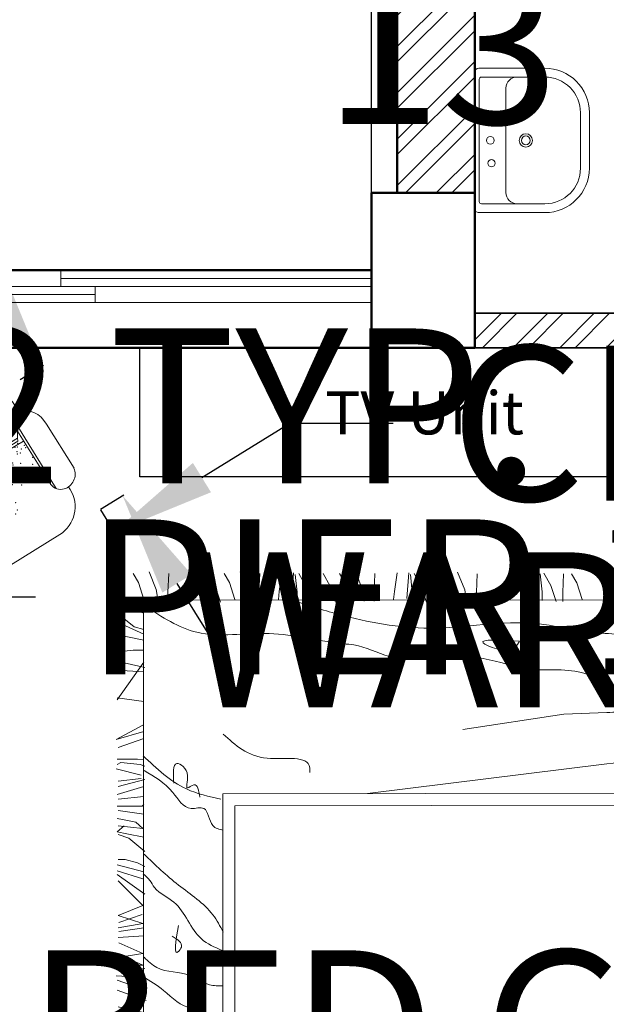
# Model space of a CAD drawing. Units: inches. Extents: x -90 to 536, y -553 to 299.
# Tile 19 of 27: x 69 to 137, y 58 to 173. Entities that reach past the tile are written whole.
import ezdxf

# ---------------------------------------------------------------- set-up
doc = ezdxf.new("R2010")
doc.units = ezdxf.units.IN
for name, color, linetype, lineweight in [('A-ANNO-DIMS', 2, 'Continuous', 18), ('A-ANNO-TEXT', 7, 'Continuous', 18), ('A-COLS', 7, 'Continuous', 50), ('A-FLOR-CASE', 2, 'Continuous', 25), ('A-FLOR-FIXT', 8, 'Continuous', 18), ('A-GLAZ', 4, 'Continuous', 18), ('A-WALL-PATT', 252, 'Continuous', 13), ('Furniture', 2, 'Continuous', 18), ('Inner Wall', 5, 'Continuous', 35), ('Outer Wall', 1, 'Continuous', 50)]:
    doc.layers.add(name, color=color, linetype=linetype, lineweight=lineweight)
doc.styles.get("Standard").update_dxf_attribs({"font": 'arial.ttf'})
doc.dimstyles.get("Standard").update_dxf_attribs({"dimtxt": 18, "dimasz": 12, "dimexe": 0.18, "dimexo": 0.0625, "dimgap": 0.09, "dimtad": 0, "dimtih": 1, "dimtoh": 1, "dimdec": 0, "dimzin": 0, "dimdsep": 46, "dimlunit": 3, "dimtxsty": 'Standard', "dimcen": 0.09, "dimadec": 0, "dimazin": 0, "dimtfac": 1, "dimtdec": 0, "dimtofl": 0, "dimtmove": 0, "dimatfit": 3, "dimfxl": 1, "dimtolj": 1, "dimtzin": 0, "dimarcsym": 0})

# ---------------------------------------------------------------- blocks, each defined once
blk = doc.blocks.new('A$C57EA129C')
for p, q in [((0, 0.4428), (0, 0.1782)), ((0.016, 0.4589), (0.5631, 0.4589)), ((0.0445, 0.441), (0.5346, 0.441)), ((0.5791, 0.4428), (0.5791, 0.1782)), ((0.0356, 0.4321), (0.0356, 0.2896)), ((0.5435, 0.4321), (0.5435, 0.2896)), ((0.0802, 0.3341), (0.499, 0.3341)), ((0.0356, 0.2896), (0.0356, 0.1782)), ((0.5435, 0.2896), (0.5435, 0.1782)), ((0.1782, 0.0356), (0.4009, 0.0356)), ((0.1782, 0), (0.4009, 0))]:
    blk.add_line(p, q)
for centre, radius in [((0.1982, 0.392), 0.0143), ((0.2896, 0.3965), 0.0156), ((0.3809, 0.392), 0.0143), ((0.2896, 0.2545), 0.0267), ((0.2896, 0.2545), 0.0178)]:
    blk.add_circle(centre, radius)
for centre, radius, start, end in [((0.016, 0.4428), 0.016, 90, 180), ((0.0445, 0.4321), 0.00891, 90, 180), ((0.5346, 0.4321), 0.00891, 0, 90), ((0.5631, 0.4428), 0.016, 0, 90), ((0.0802, 0.2896), 0.0445, 90, 180), ((0.499, 0.2896), 0.0445, 0, 90), ((0.1782, 0.1782), 0.1782, 180, 270), ((0.1782, 0.1782), 0.1426, 180, 270), ((0.4009, 0.1782), 0.1782, 270, 0), ((0.4009, 0.1782), 0.1426, 270, 0)]:
    blk.add_arc(centre, radius, start, end)
blk = doc.blocks.new('A$C14440869')
for p, q in [((299.4, 786.8), (654.5, 786.8)), ((141.1, 259.3), (141.1, 621.8)), ((154.9, 258.1), (156.1, 601.9)), ((799, 258.1), (797.7, 601.9)), ((812.8, 224.7), (812.8, 621.8)), ((0, 267.1), (1, 551.8)), ((798, 537.4), (157.2, 552.6)), ((953.9, 267.1), (952.8, 551.8)), ((78.7, 198), (78.7, 179.8)), ((875.1, 196.3), (875.2, 179.8)), ((257.3, 0.1), (696.7, 0))]:
    blk.add_line(p, q)
for centre, radius, start, end in [((178, 741.7), 84.9, 46.4058, 190.9946), ((775.9, 741.7), 84.9, 349.0054, 133.5942), ((490.5, 1647.2), 881.3, 253.2515, 257.4746), ((463.3, 1647.2), 881.3, 282.5254, 286.7485), ((146, 557.8), 145.1, 108.7163, 182.3743), ((810.8, 559.8), 142.3, 356.766, 72.1434), ((234.9, -29958.2), 30532.1, 88.98134, 90.11086), ((164.3, -28909.7), 29469.6, 88.82111, 89.96326), ((79.9, 278.7), 80.7, 188.2473, 288.8842), ((90.3, 265.5), 65, 283.9696, 353.4821), ((871.6, 268.6), 73.4, 188.2144, 251.9677), ((869.8, 281.5), 85.3, 255.8372, 350.3327), ((257.8, 179.2), 179.2, 179.795, 269.795), ((696, 179.2), 179.2, 270.205, 0.205)]:
    blk.add_arc(centre, radius, start, end)
for points in [[(94.6, 725.5), (94.6, 660.2), (167.2, 599.5), (183.2, 559.8)], [(859.3, 725.5), (859.3, 660.2), (786.7, 599.5), (770.6, 553.6)]]:
    blk.add_open_spline(points, degree=3)
for p in [(261.8, 540.6), (346.3, 540.6), (358.4, 564.7), (446.9, 540.6), (467, 548.6), (656.1, 560.7), (692.1, 540.6), (752.6, 568.7), (764.7, 544.6), (201.4, 528.5), (294, 500.4), (302, 528.5), (306.1, 524.5), (346.3, 496.4), (386.5, 484.3), (446.9, 496.4), (454.9, 524.5), (487.1, 516.5), (507.2, 520.5), (531.4, 496.4), (595.7, 520.5), (603.8, 520.5), (603.8, 484.3), (647.8, 524.5), (651.8, 528.5), (656.1, 532.5), (656.1, 524.5), (659.9, 500.4), (688.3, 492.3), (696.3, 520.5), (700.3, 528.5), (732.5, 496.4), (736.6, 508.4), (740.6, 532.5), (748.6, 492.3), (752.4, 528.5), (764.7, 508.4), (788.9, 516.5), (788.9, 500.4), (233.6, 444.1), (294, 456.2), (334.2, 444.1), (378.5, 456.2), (454.9, 480.3), (479.1, 456.2), (487.1, 440.1), (519.3, 432.1), (539.4, 480.3), (543.4, 480.3), (571.6, 472.3), (659.9, 456.2), (680.2, 456.2), (684.2, 468.2), (720.2, 444.1), (792.9, 436.1), (181.3, 403.9), (326.2, 416), (692.3, 383.9), (772.5, 403.9), (181.3, 335.6), (225.6, 339.6), (290, 339.6), (418.7, 327.6), (619.9, 367.8), (663.9, 339.6), (728.3, 339.6), (772.5, 335.6), (776.8, 339.6), (229.6, 315.5), (326.2, 303.5), (583.7, 275.4), (724.3, 315.5), (551.5, 223.1), (571.6, 235.2), (334.2, 215.1)]:
    blk.add_point(p)
blk = doc.blocks.new('A$C2B723114')
for p, q in [((0, 2.9047), (2.8274, 2.9047)), ((0, 2.8487), (0, 2.9047)), ((2.8274, 2.9047), (2.8274, 2.8487)), ((0.4243, 2.8697), (0.4243, 2.4855)), ((2.4742, 2.8697), (2.4742, 2.4855)), ((2.8274, 2.8487), (0, 2.8487)), ((0.1012, 2.4649), (0.1012, 2.849)), ((0.1396, 2.5033), (0.1396, 2.849)), ((0.6794, 0.7051), (0.6794, 2.8509)), ((0.7187, 0.7435), (0.7187, 2.8509)), ((2.1776, 2.8509), (2.1776, 0.7454)), ((2.216, 2.8509), (2.216, 0.707)), ((2.6798, 2.5052), (2.6798, 2.8509)), ((2.7182, 2.4668), (2.7182, 2.8509)), ((0.6087, 2.6776), (0.295, 2.6776)), ((2.6586, 2.6776), (2.2821, 2.6776)), ((1.3789, 2.4999), (1.3598, 2.5761)), ((2.0593, 2.4999), (2.0402, 2.5761)), ((0.6766, 2.5033), (0.1396, 2.5033)), ((1.3858, 2.4723), (1.3789, 2.4999)), ((2.0662, 2.4723), (2.0593, 2.4999)), ((2.2188, 2.5052), (2.6798, 2.5052)), ((0.6794, 2.4649), (0.1012, 2.4649)), ((0.7191, 2.47), (2.1778, 2.4719)), ((2.2188, 2.4668), (2.7182, 2.4668)), ((2.1771, 2.3036), (0.718, 2.1685)), ((1.0365, 1.6233), (2.1246, 2.2989)), ((2.2287, 1.6076), (2.2523, 1.5035)), ((0.5047, 1.5819), (0.5353, 1.4945)), ((0.6174, 1.5819), (0.6232, 1.4916)), ((0.6467, 1.5819), (0.6369, 1.5137)), ((0.6571, 1.4945), (0.6571, 1.5765)), ((2.2726, 1.593), (2.3061, 1.5007)), ((2.3067, 1.5881), (2.3373, 1.5007)), ((2.4194, 1.5881), (2.4251, 1.4979)), ((2.4487, 1.5881), (2.4389, 1.5199)), ((2.4591, 1.5007), (2.4591, 1.5828)), ((0.4269, 0.0884), (0.4269, 1.4945)), ((0.4269, 1.4945), (0.6794, 1.4945)), ((2.4685, 1.4964), (2.216, 1.5022)), ((2.4685, 1.4964), (2.4685, 0.0903)), ((0.3172, 1.3923), (0.4213, 1.3687)), ((2.4685, 1.4044), (2.5491, 1.3861)), ((2.4596, 1.3659), (2.552, 1.3324)), ((0.3318, 1.3485), (0.4241, 1.3149)), ((2.4645, 1.3318), (2.552, 1.3012)), ((0.3367, 1.3143), (0.4241, 1.2838)), ((2.4645, 1.2928), (2.5548, 1.2871)), ((2.4645, 1.2635), (2.5328, 1.2733)), ((2.4699, 1.2531), (2.552, 1.2163)), ((2.552, 1.2531), (2.4699, 1.2531)), ((2.5435, 1.2276), (2.4699, 1.2163)), ((0.3367, 1.2016), (0.427, 1.1959)), ((2.4699, 1.2163), (2.5463, 1.1823)), ((0.3367, 1.1724), (0.405, 1.1821)), ((0.4241, 1.162), (0.3421, 1.162)), ((0.3421, 1.162), (0.4241, 1.1252)), ((2.5491, 1.1654), (2.467, 1.1597)), ((2.5463, 1.1455), (2.467, 1.1342)), ((2.5491, 1.1342), (2.4699, 1.1201)), ((2.4699, 1.1201), (2.5491, 1.0946)), ((2.5463, 1.1172), (2.4727, 1.0918)), ((2.5491, 1.0946), (2.4699, 1.0635)), ((2.4699, 1.0635), (2.5491, 0.9842)), ((0.4157, 1.0206), (0.3421, 1.0093)), ((0.3421, 1.0093), (0.4185, 0.9754)), ((2.4642, 1.0267), (2.552, 0.9644)), ((2.4699, 0.9785), (2.552, 0.9531)), ((0.4213, 0.9584), (0.3392, 0.9527)), ((2.467, 0.9559), (2.552, 0.9333)), ((0.4185, 0.9386), (0.3392, 0.9272)), ((0.4213, 0.9272), (0.3421, 0.9131)), ((0.3421, 0.9131), (0.4213, 0.8876)), ((0.4185, 0.9103), (0.3449, 0.8848)), ((2.4642, 0.9389), (2.4869, 0.9276)), ((2.4869, 0.9276), (2.5265, 0.9163)), ((2.5265, 0.9163), (2.5491, 0.9163)), ((0.4213, 0.8876), (0.3421, 0.8565)), ((2.4642, 0.8908), (2.5152, 0.8483)), ((0.3421, 0.8565), (0.4213, 0.7772)), ((2.5152, 0.8483), (2.5491, 0.837)), ((0.3364, 0.8197), (0.4241, 0.7574)), ((2.467, 0.8455), (2.5208, 0.8342)), ((2.4699, 0.8172), (2.4925, 0.7974)), ((2.5491, 0.8087), (2.4699, 0.8172)), ((2.5208, 0.8342), (2.552, 0.8285)), ((2.552, 0.8285), (2.5293, 0.8087)), ((2.4925, 0.7974), (2.535, 0.7889)), ((2.535, 0.7889), (2.552, 0.7861)), ((0.3421, 0.7716), (0.4241, 0.7461)), ((2.5491, 0.7606), (2.467, 0.7719)), ((0.3392, 0.7489), (0.4241, 0.7263)), ((2.1776, 0.7454), (0.7187, 0.7435)), ((2.4727, 0.7464), (2.467, 0.7408)), ((2.467, 0.7153), (2.5491, 0.7238)), ((2.552, 0.7464), (2.4727, 0.7464)), ((0.359, 0.7206), (0.3987, 0.7093)), ((0.3987, 0.7093), (0.4213, 0.7093)), ((2.216, 0.707), (0.6794, 0.7051)), ((0.9938, 0.6115), (1.7555, 0.7064)), ((2.552, 0.7096), (2.467, 0.6842)), ((0.3421, 0.6601), (0.4213, 0.5808)), ((2.5491, 0.6842), (2.4642, 0.6615)), ((2.5491, 0.6672), (2.4755, 0.6587)), ((2.4755, 0.6474), (2.5548, 0.6276)), ((0.3364, 0.6233), (0.4241, 0.561)), ((2.4642, 0.6191), (2.4784, 0.6134)), ((2.467, 0.5993), (2.4869, 0.5964)), ((2.4784, 0.6134), (2.5406, 0.6077)), ((2.4869, 0.5964), (2.552, 0.5964)), ((2.5406, 0.6077), (2.552, 0.6134)), ((0.3421, 0.5752), (0.4241, 0.5497)), ((0.3392, 0.5525), (0.4241, 0.5299)), ((2.467, 0.5313), (2.5491, 0.5596)), ((2.467, 0.5087), (2.5548, 0.5342)), ((2.5548, 0.5342), (2.4699, 0.4889)), ((0.359, 0.5242), (0.3987, 0.5129)), ((1.4523, 0.5021), (1.1305, 0.4537)), ((0.3364, 0.4785), (0.3874, 0.436)), ((1.1305, 0.4537), (0.9938, 0.448)), ((0.4213, 0.415), (0.3364, 0.3923)), ((0.3392, 0.4332), (0.393, 0.4219)), ((0.4241, 0.2868), (0.3392, 0.415)), ((0.3874, 0.436), (0.4213, 0.4247)), ((0.393, 0.4219), (0.4241, 0.4162)), ((0.4241, 0.4162), (0.4015, 0.3964)), ((2.467, 0.4133), (2.552, 0.4019)), ((0.3421, 0.4049), (0.3647, 0.3851)), ((0.4213, 0.3964), (0.3421, 0.4049)), ((0.4213, 0.398), (0.3477, 0.3895)), ((0.3647, 0.3851), (0.4072, 0.3766)), ((0.4072, 0.3766), (0.4241, 0.3738)), ((2.467, 0.2879), (2.552, 0.4076)), ((0.4213, 0.3377), (0.3392, 0.3491)), ((0.4241, 0.3236), (0.3449, 0.3236)), ((2.467, 0.319), (2.5548, 0.3134)), ((0.3392, 0.2925), (0.4213, 0.3009)), ((2.4642, 0.3049), (2.5491, 0.2851)), ((0.3477, 0.2571), (0.427, 0.2373)), ((2.501, 0.2491), (2.5491, 0.2547)), ((0.3506, 0.2231), (0.4128, 0.2175)), ((0.4128, 0.2175), (0.4241, 0.2231)), ((2.4699, 0.2491), (2.501, 0.2491)), ((0.359, 0.2061), (0.4241, 0.2061)), ((2.467, 0.2179), (2.5605, 0.1981)), ((2.467, 0.1981), (2.5491, 0.1613)), ((2.467, 0.184), (2.4982, 0.1755)), ((2.4982, 0.1755), (2.5463, 0.1359)), ((0.3392, 0.1042), (0.4213, 0.1325)), ((2.4699, 0.1302), (2.535, 0.1104)), ((0.3392, 0.0815), (0.427, 0.107)), ((0.427, 0.107), (0.3421, 0.0617)), ((0.7334, 0.0943), (0.7503, 0.0434)), ((0.956, 0.0943), (0.973, 0.0434)), ((1.1542, 0.0943), (1.1712, 0.0434)), ((1.5674, 0.0962), (1.5844, 0.0453)), ((1.8568, 0.0962), (1.8738, 0.0453)), ((1.9342, 0.0962), (1.9512, 0.0453)), ((2.2236, 0.0962), (2.2406, 0.0453)), ((2.4642, 0.0991), (2.5378, 0.0877)), ((2.535, 0.1104), (2.5491, 0.0991)), ((2.4685, 0.0903), (0.4269, 0.0884)), ((0.5106, 0.0657), (0.5077, 0.0063)), ((0.5106, 0.094), (0.5106, 0.0657)), ((0.5417, 0.094), (0.5474, 0.0572)), ((0.587, 0.0884), (0.604, 0.0346)), ((0.6512, 0.0884), (0.6682, 0.0346)), ((0.713, 0.0657), (0.7101, 0.0063)), ((0.713, 0.094), (0.713, 0.0657)), ((0.7786, 0.0915), (0.7786, 0.0632)), ((0.7786, 0.0632), (0.7843, 0.0066)), ((0.8739, 0.0884), (0.8908, 0.0346)), ((1.0013, 0.0915), (1.0013, 0.0632)), ((1.0013, 0.0632), (1.007, 0.0066)), ((1.072, 0.0884), (1.089, 0.0346)), ((1.1338, 0.0657), (1.131, 0.0063)), ((1.1338, 0.094), (1.1338, 0.0657)), ((1.1995, 0.0915), (1.1995, 0.0632)), ((1.1995, 0.0632), (1.2052, 0.0066)), ((1.4088, 0.0657), (1.406, 0.0063)), ((1.4088, 0.094), (1.4088, 0.0657)), ((1.44, 0.094), (1.4456, 0.0572)), ((1.4853, 0.0884), (1.5023, 0.0346)), ((1.6127, 0.0934), (1.6127, 0.0651)), ((1.6127, 0.0651), (1.6184, 0.0085)), ((1.6297, 0.0849), (1.624, 0.0028)), ((1.6721, 0.0877), (1.6693, 0.0623)), ((1.7344, 0.0651), (1.7316, 0.0057)), ((1.7344, 0.0934), (1.7344, 0.0651)), ((1.7655, 0.0934), (1.7712, 0.0566)), ((1.8108, 0.0877), (1.8278, 0.034)), ((1.9795, 0.0934), (1.9795, 0.0651)), ((1.9795, 0.0651), (1.9852, 0.0085)), ((1.9965, 0.0849), (1.9908, 0.0028)), ((2.039, 0.0877), (2.0361, 0.0623)), ((2.1012, 0.0651), (2.0984, 0.0057)), ((2.1012, 0.0934), (2.1012, 0.0651)), ((2.1324, 0.0934), (2.138, 0.0566)), ((2.1777, 0.0877), (2.1946, 0.034)), ((2.2689, 0.0934), (2.2689, 0.0651)), ((2.2689, 0.0651), (2.2746, 0.0085)), ((2.2859, 0.0849), (2.2802, 0.0028)), ((2.3284, 0.0877), (2.3255, 0.0623)), ((2.3906, 0.0651), (2.3878, 0.0057)), ((2.3906, 0.0934), (2.3906, 0.0651)), ((2.4218, 0.0934), (2.4274, 0.0566)), ((2.467, 0.0877), (2.484, 0.034)), ((2.5378, 0.0877), (2.5463, 0.0821)), ((0.5474, 0.0572), (0.57, 0.0006)), ((0.604, 0.0346), (0.621, 0.0063)), ((0.6682, 0.0346), (0.6851, 0.0063)), ((0.7503, 0.0434), (0.773, 0.0037)), ((0.8908, 0.0346), (0.9078, 0.0063)), ((0.973, 0.0434), (0.9957, 0.0037)), ((1.089, 0.0346), (1.106, 0.0063)), ((1.1712, 0.0434), (1.1939, 0.0037)), ((1.4456, 0.0572), (1.4683, 0.0006)), ((1.5023, 0.0346), (1.5192, 0.0082)), ((1.5844, 0.0453), (1.607, 0.0057)), ((1.6693, 0.0623), (1.6608, 0.0028)), ((1.7712, 0.0566), (1.7938, 0)), ((1.8278, 0.034), (1.8448, 0.0057)), ((1.8738, 0.0453), (1.8964, 0.0057)), ((1.9512, 0.0453), (1.9739, 0.0057)), ((2.0361, 0.0623), (2.0276, 0.0028)), ((2.138, 0.0566), (2.1607, 0)), ((2.1946, 0.034), (2.2116, 0.0057)), ((2.2406, 0.0453), (2.2632, 0.0057)), ((2.3255, 0.0623), (2.317, 0.0028)), ((2.4274, 0.0566), (2.4501, 0)), ((2.484, 0.034), (2.501, 0.0057))]:
    blk.add_line(p, q)
for centre, radius in [((0.4243, 2.6776), 0.0821), ((2.4742, 2.6776), 0.0821), ((0.4243, 2.6776), 0.0493), ((2.4742, 2.6776), 0.0493)]:
    blk.add_circle(centre, radius)
for centre, radius, start, end in [((0.8088, 2.8207), 0.00315, 111.7883, 160.436), ((0.8162, 2.8021), 0.0232, 94.3025, 111.7883), ((0.8165, 2.7987), 0.0266, 59.3487, 94.3025), ((1.4892, 2.8207), 0.00315, 111.7883, 160.436), ((1.4966, 2.8021), 0.0232, 94.3025, 111.7883), ((1.4969, 2.7987), 0.0266, 59.3487, 94.3025), ((0.8078, 2.821), 0.00214, 160.436, 281.8931), ((0.8091, 2.8151), 0.00394, 21.9904, 101.8931), ((0.8409, 2.7949), 0.0302, 158.579, 188.1335), ((0.7994, 2.8112), 0.0144, 338.579, 21.9904), ((0.8554, 2.8643), 0.0497, 239.3487, 264.7408), ((0.9202, 3.5684), 0.7568, 264.7408, 268.0921), ((0.8679, 2.7254), 0.0915, 74.0648, 94.2159), ((0.8679, 2.7254), 0.0915, 53.9136, 74.0648), ((0.9409, 4.189), 1.3777, 268.0921, 270.5757), ((0.8679, 2.7254), 0.0915, 36.1766, 53.9136), ((0.86, 2.6097), 0.2158, 62.7604, 69.1397), ((0.9466, 3.6164), 0.8051, 270.5757, 274.8018), ((0.9263, 2.7386), 0.0708, 51.6114, 62.7604), ((0.7461, 2.511), 0.3611, 46.1885, 51.6114), ((1.0364, 2.548), 0.2671, 87.4614, 94.8018), ((1.042, 2.6745), 0.1405, 79.8101, 87.4614), ((1.1532, 3.2931), 0.488, 259.8101, 263.9133), ((1.204, 3.7695), 0.9671, 263.9133, 270), ((1.204, 3.4318), 0.6294, 270, 277.5469), ((1.2573, 3.0292), 0.2233, 277.5469, 285.744), ((1.3941, 2.5438), 0.281, 98.4372, 105.744), ((1.3747, 2.6748), 0.1486, 90, 98.4372), ((1.3713, 2.8186), 0.0315, 274.4002, 333.4195), ((1.3747, 2.74), 0.0833, 78.7276, 90), ((1.3886, 2.8099), 0.0121, 333.4195, 78.7276), ((1.4882, 2.821), 0.00214, 160.436, 281.8931), ((1.4895, 2.8151), 0.00394, 21.9904, 101.8931), ((1.5213, 2.7949), 0.0302, 158.579, 188.1335), ((1.4798, 2.8112), 0.0144, 338.579, 21.9904), ((1.5358, 2.8643), 0.0497, 239.3487, 264.7408), ((1.6006, 3.5684), 0.7568, 264.7408, 268.0921), ((1.5483, 2.7254), 0.0915, 74.0648, 94.2159), ((1.5483, 2.7254), 0.0915, 53.9136, 74.0648), ((1.6213, 4.189), 1.3777, 268.0921, 270.5757), ((1.5483, 2.7254), 0.0915, 36.1766, 53.9136), ((1.5404, 2.6097), 0.2158, 62.7604, 69.1397), ((1.627, 3.6164), 0.8051, 270.5757, 274.8018), ((1.6067, 2.7386), 0.0708, 51.6114, 62.7604), ((1.4265, 2.511), 0.3611, 46.1885, 51.6114), ((1.7168, 2.548), 0.2671, 87.4614, 94.8018), ((1.7224, 2.6745), 0.1405, 79.8101, 87.4614), ((1.8336, 3.2931), 0.488, 259.8101, 263.9133), ((1.8844, 3.7695), 0.9671, 263.9133, 270), ((1.8844, 3.4318), 0.6294, 270, 277.5469), ((1.9377, 3.0292), 0.2233, 277.5469, 285.744), ((2.0745, 2.5438), 0.281, 98.4372, 105.744), ((2.0551, 2.6748), 0.1486, 90, 98.4372), ((2.0517, 2.8186), 0.0315, 274.4002, 333.4195), ((2.0551, 2.74), 0.0833, 78.7276, 90), ((2.069, 2.8099), 0.0121, 333.4195, 78.7276), ((1.0356, 2.8227), 0.2268, 188.1335, 192.1095), ((0.635, 2.7368), 0.1829, 7.6809, 12.1095), ((-0.0181, 2.6487), 0.8418, 3.3687, 7.6809), ((0.8679, 2.7254), 0.0915, 18.4397, 36.1766), ((0.8523, 2.6218), 0.2076, 39.0349, 46.1885), ((0.923, 2.7382), 0.4535, 0, 6.2324), ((1.716, 2.8227), 0.2268, 188.1335, 192.1095), ((1.3154, 2.7368), 0.1829, 7.6809, 12.1095), ((0.6623, 2.6487), 0.8418, 3.3687, 7.6809), ((1.5483, 2.7254), 0.0915, 18.4397, 36.1766), ((1.5327, 2.6218), 0.2076, 39.0349, 46.1885), ((1.6034, 2.7382), 0.4535, 0, 6.2324), ((0.9783, 2.7239), 0.0455, 28.3168, 39.0349), ((0.8558, 2.6579), 0.1846, 23.0028, 28.3168), ((1.1884, 2.7382), 0.1881, 350.3156, 0), ((1.6587, 2.7239), 0.0455, 28.3168, 39.0349), ((1.5362, 2.6579), 0.1846, 23.0028, 28.3168), ((1.8688, 2.7382), 0.1881, 350.3156, 0), ((0.1976, 2.6614), 0.6258, 358.3669, 3.3687), ((0.5722, 2.8434), 0.8132, 347.8016, 350.3156), ((0.878, 2.6614), 0.6258, 358.3669, 3.3687), ((1.2526, 2.8434), 0.8132, 347.8016, 350.3156), ((1.6528, 2.6098), 0.2924, 167.8016, 171.9949), ((2.3332, 2.6098), 0.2924, 167.8016, 171.9949), ((-0.4351, 2.6794), 1.2587, 356.945, 358.3669), ((1.9648, 2.5659), 0.6074, 171.9949, 177.3351), ((0.2453, 2.6794), 1.2587, 356.945, 358.3669), ((2.6452, 2.5659), 0.6074, 171.9949, 177.3351), ((-11.7321, 3.2823), 12.5718, 356.49514, 356.94504), ((-11.0517, 3.2823), 12.5718, 356.49514, 356.94504), ((1.4204, 2.5912), 0.0624, 177.3351, 194.0452), ((2.1008, 2.5912), 0.0624, 177.3351, 194.0452), ((0.5206, 2.5319), 0.2961, 350.0016, 356.4951), ((1.4917, 3.1364), 0.681, 244.6889, 246.5156), ((1.4917, 3.1364), 0.681, 246.5156, 248.3423), ((1.201, 2.5319), 0.2961, 350.0016, 356.4951), ((2.1721, 3.1364), 0.681, 244.6889, 246.5156), ((2.1721, 3.1364), 0.681, 246.5156, 248.3423), ((0.8298, 2.4774), 0.0178, 170.0016, 196.6978), ((0.8068, 2.5419), 0.0707, 286.2212, 297.2841), ((0.8584, 2.4419), 0.0418, 102.869, 117.2841), ((0.879, 2.3515), 0.1345, 93.574, 102.869), ((0.9376, 1.4146), 1.0732, 90.2865, 93.574), ((0.9586, -2.7845), 5.2724, 89.0296, 90.2865), ((0.9954, -0.6123), 3.0999, 87.3904, 89.0296), ((1.0854, 1.364), 1.1216, 85.3824, 87.3904), ((1.28, 3.7729), 1.2952, 265.3824, 267.2509), ((1.228, 2.691), 0.2121, 267.2509, 281.5586), ((1.4917, 3.1364), 0.681, 248.3423, 250.572), ((1.4917, 3.1364), 0.681, 250.572, 252.8018), ((1.2975, 2.3514), 0.1345, 83.5659, 101.5586), ((1.3002, 2.3754), 0.1104, 72.6136, 83.5659), ((1.3965, 2.6828), 0.2118, 252.6136, 260.5159), ((1.5102, 2.4774), 0.0178, 170.0016, 196.6978), ((1.4872, 2.5419), 0.0707, 286.2212, 297.2841), ((1.5388, 2.4419), 0.0418, 102.869, 117.2841), ((1.5594, 2.3515), 0.1345, 93.574, 102.869), ((1.618, 1.4146), 1.0732, 90.2865, 93.574), ((1.639, -2.7845), 5.2724, 89.0296, 90.2865), ((1.6758, -0.6123), 3.0999, 87.3904, 89.0296), ((1.7658, 1.364), 1.1216, 85.3824, 87.3904), ((1.9604, 3.7729), 1.2952, 265.3824, 267.2509), ((1.9084, 2.691), 0.2121, 267.2509, 281.5586), ((2.1721, 3.1364), 0.681, 248.3423, 250.572), ((2.1721, 3.1364), 0.681, 250.572, 252.8018), ((1.9779, 2.3514), 0.1345, 83.5659, 101.5586), ((1.9806, 2.3754), 0.1104, 72.6136, 83.5659), ((2.0769, 2.6828), 0.2118, 252.6136, 260.5159), ((0.8139, 2.4726), 0.00122, 196.6978, 277.1204), ((0.8041, 2.5514), 0.0807, 277.1204, 286.2212), ((1.4027, 2.7202), 0.2496, 260.5159, 265.9171), ((1.385, 2.4721), 0.000845, 265.9171, 14.0449), ((1.4943, 2.4726), 0.00122, 196.6978, 277.1204), ((1.4845, 2.5514), 0.0807, 277.1204, 286.2212), ((2.0831, 2.7202), 0.2496, 260.5159, 265.9171), ((2.0654, 2.4721), 0.000845, 265.9171, 14.0449)]:
    blk.add_arc(centre, radius, start, end)
blk.add_ellipse((0.4962, 1.9132), major_axis=(0.4887, -0.4605), ratio=0.503305, start_param=0.491272, end_param=1.591113)
for points, knots in [([(0.6768, 1.3104), (0.6615, 1.3339), (0.6315, 1.3797), (0.604, 1.4501), (0.5417, 1.4748), (0.5064, 1.4871), (0.4848, 1.4945)], [0, 0, 0, 0, 110.980521, 216.571322, 273.316778, 363.252298, 363.252298, 363.252298, 363.252298]), ([(2.5548, 1.4853), (2.5314, 1.4757), (2.5031, 1.4641), (2.4737, 1.4555), (2.4685, 1.454)], [0, 0, 0, 0, 98.452083, 119.481049, 119.481049, 119.481049, 119.481049]), ([(0.427, 1.4678), (0.4036, 1.4582), (0.3693, 1.4441), (0.3335, 1.4344), (0.3221, 1.4313)], [0, 0, 0, 0, 98.452083, 144.639601, 144.639601, 144.639601, 144.639601]), ([(2.552, 1.4598), (2.5309, 1.4545), (2.5031, 1.4475), (2.4753, 1.4406), (2.4685, 1.4389)], [0, 0, 0, 0, 84.638756, 111.94623, 111.94623, 111.94623, 111.94623]), ([(0.4241, 1.4423), (0.4031, 1.437), (0.3691, 1.4284), (0.3351, 1.4199), (0.3221, 1.4167)], [0, 0, 0, 0, 84.638756, 136.955563, 136.955563, 136.955563, 136.955563]), ([(2.2145, 1.4211), (2.233, 1.4246), (2.2636, 1.4303), (2.2761, 1.3837), (2.3429, 1.3967), (2.3949, 1.3342), (2.4474, 1.3031), (2.4698, 1.2898)], [0, 0, 0, 0, 61.886907, 102.717887, 145.699352, 284.082577, 386.765171, 386.765171, 386.765171, 386.765171]), ([(0.6768, 1.286), (0.6567, 1.2911), (0.6145, 1.3017), (0.5543, 1.3533), (0.4816, 1.349), (0.4362, 1.3493), (0.4233, 1.3493)], [0, 0, 0, 0, 80.250278, 168.388677, 295.908361, 346.663112, 346.663112, 346.663112, 346.663112]), ([(0.4233, 1.3445), (0.4367, 1.3385), (0.464, 1.3264), (0.5129, 1.2848), (0.5456, 1.2161), (0.6131, 1.2349), (0.6142, 1.1913), (0.6642, 1.1806), (0.674, 1.144), (0.6817, 1.1154)], [0, 0, 0, 0, 56.745495, 115.23739, 254.956954, 286.678662, 337.828324, 366.201072, 468.500395, 468.500395, 468.500395, 468.500395]), ([(2.2145, 1.319), (2.2295, 1.319), (2.2678, 1.3192), (2.3288, 1.2705), (2.4143, 1.279), (2.4535, 1.2403), (2.4662, 1.2278)], [0, 0, 0, 0, 57.155505, 146.33427, 287.936209, 355.396728, 355.396728, 355.396728, 355.396728]), ([(2.3573, 1.127), (2.3656, 1.1759), (2.3758, 1.2352), (2.3371, 1.1853), (2.3602, 1.1713), (2.3768, 1.1612)], [0, 0, 0, 0, 107.853607, 130.728419, 189.220329, 189.220329, 189.220329, 189.220329]), ([(2.2182, 1.2059), (2.2419, 1.1958), (2.3116, 1.1659), (2.342, 1.0552), (2.4266, 1.0223), (2.4474, 0.9811), (2.462, 0.9684), (2.4698, 0.9616)], [0, 0, 0, 0, 97.73655, 287.59661, 389.176293, 423.403759, 463.679181, 463.679181, 463.679181, 463.679181]), ([(2.2145, 1.1476), (2.2246, 1.1286), (2.2575, 1.0666), (2.3612, 1.0009), (2.431, 0.9336), (2.4662, 0.8996)], [0, 0, 0, 0, 83.02987, 271.460712, 463.033803, 463.033803, 463.033803, 463.033803]), ([(0.6817, 0.8034), (0.6673, 0.8119), (0.6341, 0.8315), (0.5785, 0.8518), (0.5349, 0.8973), (0.4828, 0.9461), (0.4518, 0.9879), (0.4331, 1.013)], [0, 0, 0, 0, 65.318952, 150.437229, 226.833166, 307.58338, 429.454095, 429.454095, 429.454095, 429.454095]), ([(0.4282, 0.9448), (0.4547, 0.9353), (0.496, 0.9206), (0.5223, 0.8436), (0.5628, 0.7946), (0.6113, 0.7575), (0.6214, 0.7173), (0.6539, 0.7022), (0.672, 0.6897), (0.6768, 0.6864)], [0, 0, 0, 0, 102.299436, 159.044876, 303.717955, 348.579152, 391.138254, 454.581655, 477.456496, 477.456496, 477.456496, 477.456496]), ([(2.2145, 0.823), (2.227, 0.8201), (2.261, 0.8121), (2.261, 0.7401), (2.3352, 0.7659), (2.379, 0.6836), (2.4336, 0.6521), (2.4662, 0.6334)], [0, 0, 0, 0, 46.747668, 127.438174, 179.649794, 280.561838, 429.605131, 429.605131, 429.605131, 429.605131]), ([(0.4282, 0.74), (0.4347, 0.7029), (0.444, 0.6496), (0.5194, 0.6274), (0.555, 0.5807), (0.5975, 0.5243), (0.6789, 0.5415), (0.677, 0.5095), (0.6768, 0.5061)], [0, 0, 0, 0, 130.791737, 187.537266, 286.231946, 353.673191, 460.023761, 472.712403, 472.712403, 472.712403, 472.712403]), ([(2.2218, 0.7246), (2.2595, 0.716), (2.3548, 0.6945), (2.4265, 0.6268), (2.4698, 0.586)], [0, 0, 0, 0, 148.665024, 375.555892, 375.555892, 375.555892, 375.555892]), ([(2.3719, 0.6737), (2.3738, 0.6431), (2.3772, 0.5878), (2.3146, 0.6382), (2.3401, 0.7015), (2.2971, 0.6649), (2.2923, 0.6965), (2.289, 0.7176)], [0, 0, 0, 0, 83.446591, 150.887818, 201.642461, 230.015204, 286.760644, 286.760644, 286.760644, 286.760644]), ([(0.6768, 0.6864), (0.7275, 0.655), (0.8251, 0.5944), (0.9391, 0.606), (0.9938, 0.6115)], [0, 0, 0, 0, 225.995823, 434.686543, 434.686543, 434.686543, 434.686543]), ([(2.2145, 0.5167), (2.1764, 0.5522), (2.1051, 0.6184), (1.9357, 0.5803), (1.9385, 0.6342), (1.9388, 0.6395)], [0, 0, 0, 0, 208.073343, 389.01094, 409.01094, 409.01094, 409.01094, 409.01094]), ([(0.6768, 0.5061), (0.7554, 0.4794), (0.8591, 0.4442), (0.9675, 0.4473), (0.9938, 0.448)], [0, 0, 0, 0, 319.374611, 421.61723, 421.61723, 421.61723, 421.61723]), ([(0.4331, 0.4427), (0.4498, 0.4356), (0.4827, 0.4216), (0.5314, 0.3759), (0.632, 0.3884), (0.6996, 0.3513), (0.7423, 0.3278)], [0, 0, 0, 0, 70.931849, 139.556414, 248.154027, 434.709995, 434.709995, 434.709995, 434.709995]), ([(2.4625, 0.1088), (2.4095, 0.1438), (2.2904, 0.2226), (2.0623, 0.1771), (1.9006, 0.2246), (1.7699, 0.2337), (1.6941, 0.2766), (1.5528, 0.2786), (1.4005, 0.2587), (1.2324, 0.3267), (1.059, 0.2939), (0.9218, 0.426), (0.7359, 0.3204), (0.5586, 0.2391), (0.4502, 0.3116), (0.427, 0.3272)], [0, 0, 0, 0, 239.874704, 538.942419, 850.40885, 893.390315, 1047.998294, 1176.505142, 1437.500972, 1637.333004, 1864.324391, 2089.058767, 2248.736533, 2637.953392, 2744.252142, 2744.252142, 2744.252142, 2744.252142]), ([(1.9771, 0.0962), (1.9286, 0.1117), (1.7864, 0.157), (1.5223, 0.1992), (1.2611, 0.141), (1.0527, 0.2023), (0.8859, 0.1885), (0.76, 0.3042), (0.6211, 0.292), (0.5187, 0.3203), (0.4572, 0.3456), (0.4282, 0.3575)], [0, 0, 0, 0, 198.710624, 582.73994, 1031.873213, 1206.082894, 1423.278209, 1655.952104, 1808.744089, 1945.69963, 2068.229211, 2068.229211, 2068.229211, 2068.229211]), ([(0.8718, 0.2941), (0.8821, 0.3221), (0.9041, 0.3814), (0.9523, 0.2773), (0.8733, 0.2454), (0.8757, 0.2798), (0.8766, 0.2941)], [0, 0, 0, 0, 82.720021, 175.094899, 237.579423, 282.440623, 282.440623, 282.440623, 282.440623]), ([(0.8474, 0.0943), (0.82, 0.1047), (0.757, 0.1287), (0.6201, 0.1029), (0.4623, 0.1837), (0.4372, 0.2936), (0.4282, 0.3331)], [0, 0, 0, 0, 112.422038, 258.341957, 533.791494, 688.286079, 688.286079, 688.286079, 688.286079]), ([(1.2715, 0.221), (1.3344, 0.2172), (1.4529, 0.21), (1.2971, 0.2665), (1.2756, 0.2284), (1.2715, 0.221)], [0, 0, 0, 0, 150.888188, 283.977876, 315.699589, 315.699589, 315.699589, 315.699589])]:
    blk.add_open_spline(points, degree=3, knots=knots)
blk = doc.blocks.new('COL-12X18')
blk.add_lwpolyline([(0, 18), (12, 18), (12, 0), (0, 0)], close=True)
blk = doc.blocks.new('TV-UNIT')
blk.add_lwpolyline([(15, 65.77), (15, 0), (0, 0), (0, 65.77)], close=True)
blk = doc.blocks.new('*D26')
at = {"layer": 'A-ANNO-DIMS', "color": 0, "lineweight": -2, "transparency": 16777216}
for p, q in [((201.13, 169.45), (189.13, 169.45)), ((213.13, 167), (213.13, 169.63)), ((226.43, 167), (226.43, 169.63)), ((238.43, 169.45), (250.43, 169.45))]:
    blk.add_line(p, q, dxfattribs=at)
at = {"layer": 'A-ANNO-DIMS', "color": 0, "transparency": 16777216}
for points in [[(201.13, 171.45), (201.13, 167.45), (213.13, 169.45)], [(238.43, 171.45), (238.43, 167.45), (226.43, 169.45)]]:
    blk.add_solid(points, dxfattribs=at)
at = {"layer": 'Defpoints', "color": 0, "transparency": 16777216}
for p in [(213.13, 169.45), (213.13, 166.94), (226.43, 166.94)]:
    blk.add_point(p, dxfattribs=at)
at = {"layer": 'A-ANNO-DIMS', "color": 0, "transparency": 16777216, "insert": (146.08, 169.45), "char_height": 18, "attachment_point": 5}
blk.add_mtext('\\A1;13 TYP.', dxfattribs=at)
blk = doc.blocks.new('*D31')
at = {"layer": 'A-ANNO-DIMS', "color": 0, "lineweight": -2, "transparency": 16777216}
for p, q in [((90.45, 119.36), (100.65, 125.67)), ((100.65, 125.67), (112.65, 125.67)), ((78.67, 115.59), (80.34, 112.89)), ((61.33, 104.86), (63, 102.15)), ((52.7, 95.99), (42.5, 89.68))]:
    blk.add_line(p, q, dxfattribs=at)
at = {"layer": 'A-ANNO-DIMS', "color": 0, "transparency": 16777216}
for points in [[(89.4, 121.06), (91.5, 117.65), (80.24, 113.04)], [(51.65, 97.69), (53.76, 94.29), (62.91, 102.31)]]:
    blk.add_solid(points, dxfattribs=at)
at = {"layer": 'Defpoints', "color": 0, "transparency": 16777216}
for p in [(78.63, 115.64), (80.24, 113.04), (61.3, 104.91)]:
    blk.add_point(p, dxfattribs=at)
at = {"layer": 'A-ANNO-DIMS', "color": 0, "transparency": 16777216, "insert": (199.06, 125.67), "char_height": 18, "attachment_point": 5}
blk.add_mtext('\\A1;CHAIR 20 TYP.', dxfattribs=at)
blk = doc.blocks.new('*D32')
at = {"layer": 'A-ANNO-DIMS', "color": 0, "lineweight": -2, "transparency": 16777216}
for p, q in [((59.26, 152.75), (47.26, 152.75)), ((65.58, 142.54), (59.26, 152.75)), ((69.35, 130.76), (72.05, 132.44)), ((78.69, 115.67), (81.39, 117.34)), ((87.55, 107.05), (93.87, 96.84))]:
    blk.add_line(p, q, dxfattribs=at)
at = {"layer": 'A-ANNO-DIMS', "color": 0, "transparency": 16777216}
for points in [[(67.28, 143.6), (63.88, 141.49), (71.89, 132.34)], [(89.25, 108.1), (85.85, 105.99), (81.24, 117.25)]]:
    blk.add_solid(points, dxfattribs=at)
at = {"layer": 'Defpoints', "color": 0, "transparency": 16777216}
for p in [(71.89, 132.34), (69.29, 130.73), (78.63, 115.64)]:
    blk.add_point(p, dxfattribs=at)
at = {"layer": 'A-ANNO-DIMS', "color": 0, "transparency": 16777216, "insert": (4.21, 152.75), "char_height": 18, "attachment_point": 5}
blk.add_mtext('\\A1;18 TYP.', dxfattribs=at)
blk = doc.blocks.new('*D33')
at = {"layer": 'A-ANNO-DIMS', "color": 0, "lineweight": -2, "transparency": 16777216}
for p, q in [((173.76, 108.4), (189.77, 108.4)), ((189.59, 96.4), (189.59, 64.83)), ((189.59, 14.45), (189.59, 46.02)), ((173.76, 2.45), (189.77, 2.45))]:
    blk.add_line(p, q, dxfattribs=at)
at = {"layer": 'A-ANNO-DIMS', "color": 0, "transparency": 16777216}
for points in [[(187.59, 96.4), (191.59, 96.4), (189.59, 108.4)], [(187.59, 14.45), (191.59, 14.45), (189.59, 2.45)]]:
    blk.add_solid(points, dxfattribs=at)
at = {"layer": 'Defpoints', "color": 0, "transparency": 16777216}
for p in [(173.7, 108.4), (173.7, 2.45), (189.59, 2.45)]:
    blk.add_point(p, dxfattribs=at)
at = {"layer": 'A-ANNO-DIMS', "color": 0, "transparency": 16777216, "insert": (189.59, 55.42), "char_height": 18, "attachment_point": 5}
blk.add_mtext('\\A1;BED GROUP 106 TYP.', dxfattribs=at)
blk = doc.blocks.new('*D37')
at = {"layer": 'A-ANNO-DIMS', "color": 0, "lineweight": -2, "transparency": 16777216}
for p, q in [((23.09, 105.5), (11.09, 105.5)), ((35.09, 103.75), (35.09, 105.68)), ((47.13, 103.75), (47.13, 105.68)), ((59.13, 105.5), (71.13, 105.5))]:
    blk.add_line(p, q, dxfattribs=at)
at = {"layer": 'A-ANNO-DIMS', "color": 0, "transparency": 16777216}
for points in [[(23.09, 107.5), (23.09, 103.5), (35.09, 105.5)], [(59.13, 107.5), (59.13, 103.5), (47.13, 105.5)]]:
    blk.add_solid(points, dxfattribs=at)
at = {"layer": 'Defpoints', "color": 0, "transparency": 16777216}
for p in [(47.13, 105.5), (35.09, 103.69), (47.13, 103.69)]:
    blk.add_point(p, dxfattribs=at)
at = {"layer": 'A-ANNO-DIMS', "color": 0, "transparency": 16777216, "insert": (147.42, 105.5), "char_height": 18, "attachment_point": 5}
blk.add_mtext('\\A1;PIER 12 TYP.', dxfattribs=at)
blk = doc.blocks.new('*D38')
at = {"layer": 'A-ANNO-DIMS', "color": 0, "lineweight": -2, "transparency": 16777216}
for p, q in [((33.28, 115.69), (33.28, 127.69)), ((33.28, 127.69), (45.28, 127.69)), ((35.02, 103.69), (33.1, 103.69)), ((35.02, 91.93), (33.1, 91.93)), ((33.28, 79.93), (33.28, 67.93))]:
    blk.add_line(p, q, dxfattribs=at)
at = {"layer": 'A-ANNO-DIMS', "color": 0, "transparency": 16777216}
for points in [[(31.28, 115.69), (35.28, 115.69), (33.28, 103.69)], [(31.28, 79.93), (35.28, 79.93), (33.28, 91.93)]]:
    blk.add_solid(points, dxfattribs=at)
at = {"layer": 'Defpoints', "color": 0, "transparency": 16777216}
for p in [(33.28, 103.69), (35.09, 103.69), (35.09, 91.93)]:
    blk.add_point(p, dxfattribs=at)
at = {"layer": 'A-ANNO-DIMS', "color": 0, "transparency": 16777216, "insert": (88.33, 127.69), "char_height": 18, "attachment_point": 5}
blk.add_mtext('\\A1;12 TYP.', dxfattribs=at)
blk = doc.blocks.new('*D39')
at = {"layer": 'A-ANNO-DIMS', "color": 0, "lineweight": -2, "transparency": 16777216}
for p, q in [((209.07, 134.45), (199.12, 134.45)), ((199.3, 122.45), (199.3, 111.07)), ((199.3, 80.89), (199.3, 92.26)), ((209.07, 68.89), (199.12, 68.89))]:
    blk.add_line(p, q, dxfattribs=at)
at = {"layer": 'A-ANNO-DIMS', "color": 0, "transparency": 16777216}
for points in [[(197.3, 122.45), (201.3, 122.45), (199.3, 134.45)], [(197.3, 80.89), (201.3, 80.89), (199.3, 68.89)]]:
    blk.add_solid(points, dxfattribs=at)
at = {"layer": 'Defpoints', "color": 0, "transparency": 16777216}
for p in [(199.3, 134.45), (209.13, 134.45), (209.13, 68.89)]:
    blk.add_point(p, dxfattribs=at)
at = {"layer": 'A-ANNO-DIMS', "color": 0, "transparency": 16777216, "insert": (199.3, 101.67), "char_height": 18, "attachment_point": 5}
blk.add_mtext('\\A1;WARDROBE 66 TYP.', dxfattribs=at)
blk = doc.blocks.new('*D53')
at = {"layer": 'A-ANNO-DIMS', "color": 0, "lineweight": -2, "transparency": 16777216}
for p, q in [((35.09, 103.75), (35.09, 287.38)), ((407.13, -63.49), (407.13, 287.38)), ((47.09, 287.2), (183.7, 287.2)), ((395.13, 287.2), (258.52, 287.2))]:
    blk.add_line(p, q, dxfattribs=at)
at = {"layer": 'A-ANNO-DIMS', "color": 0, "transparency": 16777216}
for points in [[(47.09, 289.2), (47.09, 285.2), (35.09, 287.2)], [(395.13, 289.2), (395.13, 285.2), (407.13, 287.2)]]:
    blk.add_solid(points, dxfattribs=at)
at = {"layer": 'Defpoints', "color": 0, "transparency": 16777216}
for p in [(407.13, 287.2), (35.09, 103.69), (407.13, -63.55)]:
    blk.add_point(p, dxfattribs=at)
at = {"layer": 'A-ANNO-DIMS', "color": 0, "transparency": 16777216, "insert": (221.11, 287.2), "char_height": 18, "attachment_point": 5}
blk.add_mtext('\\A1;372.04', dxfattribs=at)
blk = doc.blocks.new('*D54')
at = {"layer": 'A-ANNO-DIMS', "color": 0, "lineweight": -2, "transparency": 16777216}
for p, q in [((113.07, 249.45), (-2.85, 249.45)), ((-2.67, 237.45), (-2.67, -117.77)), ((-2.67, -491.55), (-2.67, -136.34)), ((38.07, -503.55), (-2.85, -503.55))]:
    blk.add_line(p, q, dxfattribs=at)
at = {"layer": 'A-ANNO-DIMS', "color": 0, "transparency": 16777216}
for points in [[(-4.67, 237.45), (-0.67, 237.45), (-2.67, 249.45)], [(-4.67, -491.55), (-0.67, -491.55), (-2.67, -503.55)]]:
    blk.add_solid(points, dxfattribs=at)
at = {"layer": 'Defpoints', "color": 0, "transparency": 16777216}
for p in [(-2.67, 249.45), (113.13, 249.45), (38.13, -503.55)]:
    blk.add_point(p, dxfattribs=at)
at = {"layer": 'A-ANNO-DIMS', "color": 0, "transparency": 16777216, "insert": (-2.67, -127.05), "char_height": 18, "attachment_point": 5}
blk.add_mtext('\\A1;753', dxfattribs=at)
blk = doc.blocks.new('*D63')
at = {"layer": 'A-ANNO-DIMS', "color": 0, "lineweight": -2, "transparency": 16777216}
for p, q in [((38.13, 143.51), (38.13, 287.38)), ((110.13, 143.51), (110.13, 287.38)), ((50.13, 287.2), (61.32, 287.2)), ((98.13, 287.2), (86.95, 287.2))]:
    blk.add_line(p, q, dxfattribs=at)
at = {"layer": 'A-ANNO-DIMS', "color": 0, "transparency": 16777216}
for points in [[(50.13, 289.2), (50.13, 285.2), (38.13, 287.2)], [(98.13, 289.2), (98.13, 285.2), (110.13, 287.2)]]:
    blk.add_solid(points, dxfattribs=at)
at = {"layer": 'Defpoints', "color": 0, "transparency": 16777216}
for p in [(110.13, 287.2), (38.13, 143.45), (110.13, 143.45)]:
    blk.add_point(p, dxfattribs=at)
at = {"layer": 'A-ANNO-DIMS', "color": 0, "transparency": 16777216, "insert": (74.13, 287.2), "char_height": 18, "attachment_point": 5}
blk.add_mtext('\\A1;72', dxfattribs=at)

msp = doc.modelspace()

# ---------------------------------------------------------------- hatches: boundary and pattern name
at = {"layer": 'A-WALL-PATT'}
h = msp.add_hatch(dxfattribs=at)
h.set_pattern_fill('ANSI32', color=256, scale=0.4)
h.set_pattern_definition([(45, (-88.8105, -603.6155), (-2.694077, 2.694077), []), (45, (-87.0145, -603.6155), (-2.694077, 2.694077), [])])
h.paths.add_polyline_path([(285.1317, 246.4462), (131.1317, 246.4462), (131.1317, 237.4462), (285.1317, 237.4462)])
h.paths.add_polyline_path([(122.1317, 237.4462), (113.1317, 237.4462), (113.1317, 152.4462), (122.1317, 152.4462), (122.1317, 166.4704)])
h.paths.add_polyline_path([(303.1317, 237.4462), (294.1317, 237.4462), (294.1317, 152.4462), (303.1317, 152.4462)])
h.paths.add_polyline_path([(47.1317, 91.9277), (38.1317, 91.9277), (38.1317, -6.5538), (77.1317, -6.5538), (77.1317, 2.4462), (70.5655, 2.4462), (47.1317, 2.4462)])
h.paths.add_polyline_path([(83.052, -61.5538), (47.1317, -61.5538), (47.1317, -24.5538), (38.1317, -24.5538), (38.1317, -70.5538), (74.052, -70.5538), (74.052, -223.5538), (38.1317, -223.5538), (38.1317, -503.5538), (92.1317, -503.5538), (92.1317, -437.5538), (191.1317, -437.5538), (191.1317, -428.5538), (83.1317, -428.5538), (83.1317, -494.5538), (47.1317, -494.5538), (47.1317, -232.5538), (83.052, -232.5538), (83.052, -70.5538)])
h.paths.add_polyline_path([(407.1317, -63.5538), (381.1317, -63.5538), (381.1317, 91.9277), (372.1317, 91.9277), (372.1317, 32.8805), (372.1317, -63.5538), (306.5745, -63.5538), (237.1317, -63.5538), (237.1317, -38.5538), (233.1317, -38.5538), (233.1317, -71.5538), (398.1317, -71.5538), (398.1317, -152.5538), (233.1317, -152.5538), (233.1317, -161.5538), (398.1317, -161.5538), (398.1317, -368.5538), (233.1317, -368.5538), (233.1317, -377.5538), (407.1317, -377.5538), (407.1317, -161.5538)])
h.paths.add_polyline_path([(261.1317, -422.5538), (252.1317, -422.5538), (252.1317, -428.5538), (233.1317, -428.5538), (233.1317, -437.5538), (261.1317, -437.5538)])
h.paths.add_polyline_path([(191.1317, -368.5538), (180.1317, -368.5538), (180.1317, -335.5538), (131.5919, -335.5538), (131.5919, -344.5538), (171.1317, -344.5538), (171.1317, -392.5538), (180.1317, -392.5538), (180.1317, -377.5538), (191.1317, -377.5538)], flags=17)
h.paths.add_polyline_path([(180.1317, -223.5538), (152.1317, -223.5538), (152.1317, -227.5538), (176.1317, -227.5538), (176.1317, -335.5538), (180.1317, -335.5538)], flags=17)
h.paths.add_polyline_path([(131.5919, -335.5538), (83.1317, -335.5538), (83.1317, -339.5538), (83.1317, -392.5538), (87.1317, -392.5538), (87.1317, -339.5538), (131.5919, -339.5538)], flags=17)
h.paths.add_polyline_path([(197.1317, 2.4462), (77.1317, 2.4462), (77.1317, -1.5538), (113.1317, -1.5538), (113.1317, -71.5538), (181.1317, -71.5538), (181.1317, -67.5538), (117.1317, -67.5538), (117.1317, -1.5538), (177.1317, -1.5538), (177.1317, -37.5538), (181.1317, -37.5538), (181.1317, -1.5538), (197.1317, -1.5538)])
h.paths.add_polyline_path([(173.1317, 138.4462), (122.1317, 138.4462), (122.1317, 134.4462), (173.1317, 134.4462)])
h.paths.add_polyline_path([(213.1317, 237.4462), (209.1317, 237.4462), (209.1317, 134.4462), (233.1317, 134.4462), (233.1317, 68.8889), (233.1317, -2.5538), (237.1317, -2.5538), (237.1317, 134.4462), (258.1317, 134.4462), (258.1317, 138.4462), (213.1317, 138.4462)])

# ---------------------------------------------------------------- linework, layer by layer
at = {"layer": 'A-GLAZ'}
for p, q in [((74.0545, 142.5076), (110.1317, 142.5076)), ((41.9772, 140.6303), (78.0545, 140.6303)), ((76.0545, 139.6916), (110.1317, 139.6916))]:
    msp.add_line(p, q, dxfattribs=at)
for points in [[(74.0545, 141.5689), (110.1317, 141.5689), (110.1317, 143.4462), (74.0545, 143.4462)], [(41.9772, 139.6916), (78.0545, 139.6916), (78.0545, 141.5689), (41.9772, 141.5689)]]:
    msp.add_lwpolyline(points, close=True, dxfattribs=at)
at = {"layer": 'Inner Wall'}
for p, q in [((173.1317, 138.4462), (122.1317, 138.4462)), ((173.1317, 134.4462), (122.1317, 134.4462))]:
    msp.add_line(p, q, dxfattribs=at)
at = {"layer": 'Outer Wall'}
for p, q in [((113.1317, 152.4462), (113.1317, 246.4462)), ((122.1317, 138.4462), (122.1317, 237.4462)), ((110.1317, 143.4462), (38.1317, 143.4462)), ((110.1317, 134.4462), (47.1317, 134.4462))]:
    msp.add_line(p, q, dxfattribs=at)

# ---------------------------------------------------------------- block references
at = {"layer": 'A-COLS'}
msp.add_blockref('COL-12X18', (110.1317, 134.4462), dxfattribs=at)
at = {"layer": 'A-FLOR-CASE', "rotation": 90.00000000000007}
msp.add_blockref('TV-UNIT', (149.0162, 119.4462), dxfattribs=at)
at = {"layer": 'A-FLOR-FIXT', "xscale": 28.98333223671166, "yscale": 28.98333223671166, "zscale": 28.98333223671166, "rotation": 89.99999999999999}
msp.add_blockref('A$C57EA129C', (135.4312, 150.1495), dxfattribs=at)
at = {"layer": 'Furniture'}
for name, p, xscale, yscale, zscale, rotation in [('A$C14440869', (61.3263, 104.927), 0.0212813664299499, 0.0212813664299499, 0.0212813664299499, 31.75670152915393), ('A$C2B723114', (173.698, 108.4009), 36.47664764473289, 36.47664764473289, 36.47664764473289, 180)]:
    msp.add_blockref(name, p, dxfattribs=dict(at, xscale=xscale, yscale=yscale, zscale=zscale, rotation=rotation))

# ---------------------------------------------------------------- texts
at = {"layer": 'A-ANNO-TEXT', "insert": (133.9175, 129.3768), "char_height": 5, "attachment_point": 3}
msp.add_mtext_dynamic_manual_height_columns('\\pxqc;{\\fTimes New Roman|b0|i0|c0|p18;TV Unit}', width=35.23368, gutter_width=12.5, heights=[0], dxfattribs=at)

# ---------------------------------------------------------------- dimensions: what is measured, and where the dimension line sits
at = {"layer": 'A-ANNO-DIMS'}
for base, p1, p2, override, picture, middle in [((407.1317, 287.2012), (35.0873, 103.6916), (407.1317, -63.5538), {"dimdec": 2, "dimlfac": 1, "dimrnd": 0, "dimzin": 0, "dimdsep": 46, "dimlunit": 2}, '*D53', (221.1095, 287.2012)), ((110.1317, 287.2012), (38.1317, 143.4462), (110.1317, 143.4462), {"dimdec": 0, "dimlfac": 1, "dimrnd": 0, "dimzin": 0, "dimdsep": 46, "dimlunit": 2}, '*D63', (74.1317, 287.2012))]:
    dim = msp.add_linear_dim(base=base, p1=p1, p2=p2, dimstyle='Standard', override=override, dxfattribs=at)
    dim.commit()
    dim.dimension.update_dxf_attribs({"geometry": picture, "text_midpoint": middle})
dim = msp.add_linear_dim(base=(-2.6677, 249.4462), p1=(38.1317, -503.5538), p2=(113.1317, 249.4462), angle=90, dimstyle='Standard', override={"dimdec": 0, "dimlfac": 1, "dimrnd": 0, "dimzin": 0, "dimdsep": 46, "dimlunit": 2}, dxfattribs=at)
dim.commit()
dim.dimension.update_dxf_attribs({"geometry": '*D54', "text_midpoint": (-2.6677, -127.0538)})
for base, p1, p2, angle, text, picture, middle in [((213.1317, 169.4531), (226.4312, 166.9352), (213.1317, 166.9352), 180, '<> TYP.', '*D26', (146.0799, 169.4531)), ((71.8939, 132.3414), (78.6344, 115.6404), (69.2932, 130.7316), 121.756702, '<> TYP.', '*D32', (4.2106, 152.7484)), ((80.2442, 113.0397), (61.2964, 104.9085), (78.6344, 115.6404), 31.756702, 'CHAIR <> TYP.', '*D31', (199.0577, 125.6712)), ((33.2806, 103.6916), (35.0873, 91.9277), (35.0873, 103.6916), 90, '<> TYP.', '*D38', (88.3324, 127.6916)), ((199.2981, 134.4462), (209.1317, 68.8889), (209.1317, 134.4462), 90, 'WARDROBE <> TYP.', '*D39', (199.2981, 101.6676)), ((189.5912, 2.4462), (173.698, 108.4009), (173.698, 2.4462), 270, 'BED GROUP <> TYP.', '*D33', (189.5912, 55.4235))]:
    dim = msp.add_linear_dim(base=base, p1=p1, p2=p2, angle=angle, text=text, dimstyle='Standard', override={"dimdec": 0, "dimlfac": 1, "dimrnd": 0, "dimzin": 0, "dimdsep": 46, "dimlunit": 2}, dxfattribs=at)
    dim.commit()
    dim.dimension.update_dxf_attribs({"geometry": picture, "text_midpoint": middle})
dim = msp.add_linear_dim(base=(47.1317, 105.4983), p1=(35.0873, 103.6916), p2=(47.1317, 103.6916), text='PIER <> TYP.', dimstyle='Standard', override={"dimdec": 0, "dimlfac": 1, "dimrnd": 0, "dimzin": 0, "dimdsep": 46, "dimlunit": 2}, dxfattribs=at)
dim.commit()
dim.dimension.update_dxf_attribs({"geometry": '*D37', "text_midpoint": (147.4209, 105.4983)})

doc.saveas('drawing.dxf')
